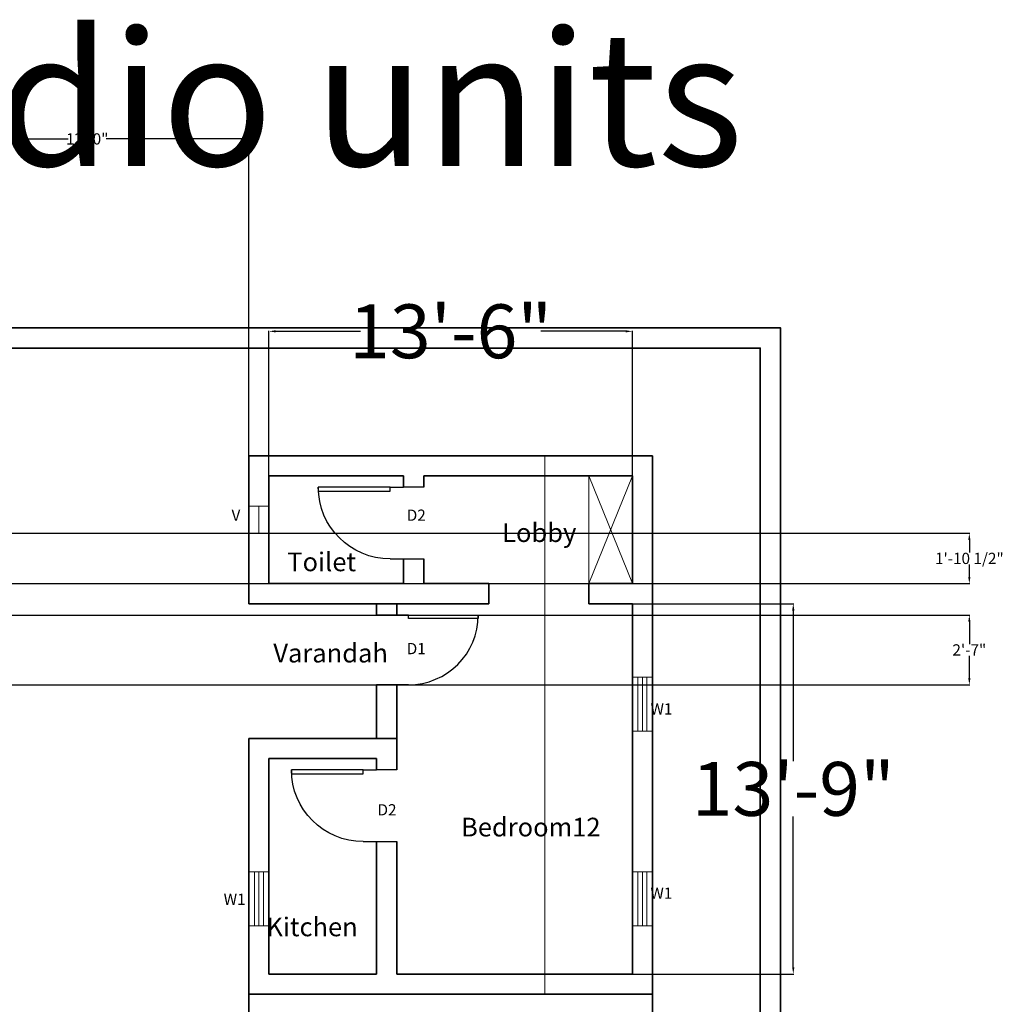
# Model space of a CAD drawing. Units: inches. Extents: x -205 to 674, y 63 to 1798.
# Tile 4 of 4: x 236 to 674, y 1359 to 1798. Entities that reach past the tile are written whole.
import ezdxf

# ---------------------------------------------------------------- set-up
doc = ezdxf.new("R2010")
doc.units = ezdxf.units.IN
doc.header["$MEASUREMENT"] = 0
doc.layers.get('0').update_dxf_attribs({"color": 70})
for name, color, linetype, lineweight in [('A-ANNO-DIMS', 240, 'Continuous', 18), ('A-ANNO-TEXT', 240, 'Continuous', 18), ('A-AREA-IDEN', 240, 'Continuous', 18), ('A-REFR', 8, 'Continuous', 13), ('A-WALL', 70, 'Continuous', 35), ('A-WALL-SITE', 70, 'Continuous', 35), ('door1', 20, 'Continuous', 25), ('door2', 160, 'Continuous', 25), ('lobby', 241, 'Continuous', 18), ('ventilator1', 210, 'Continuous', 18), ('window1', 50, 'Continuous', 18)]:
    doc.layers.add(name, color=color, linetype=linetype, lineweight=lineweight)
doc.styles.get("Standard").update_dxf_attribs({"font": 'arial.ttf'})
doc.dimstyles.get("Standard").update_dxf_attribs({"dimtxt": 5, "dimasz": 3, "dimexe": 0.18, "dimexo": 0.0625, "dimgap": 0.09, "dimtad": 0, "dimtih": 1, "dimtoh": 1, "dimdec": 0, "dimzin": 0, "dimdsep": 46, "dimlunit": 3, "dimtxsty": 'Standard', "dimcen": 0.09, "dimadec": 0, "dimazin": 0, "dimtfac": 1, "dimtdec": 0, "dimtofl": 0, "dimtmove": 0, "dimatfit": 3, "dimfxl": 1, "dimtolj": 1, "dimtzin": 0, "dimarcsym": 0})

# ---------------------------------------------------------------- blocks, each defined once
blk = doc.blocks.new('*D16')
at = {"layer": 'A-ANNO-DIMS', "color": 0, "lineweight": -2, "transparency": 16777216}
for p, q in [((509.6, 1537.3), (581.44, 1537.3)), ((581.26, 1534.3), (581.26, 1467.15)), ((581.26, 1375.3), (581.26, 1442.45)), ((509.6, 1372.3), (581.44, 1372.3))]:
    blk.add_line(p, q, dxfattribs=at)
at = {"layer": 'A-ANNO-DIMS', "color": 0, "transparency": 16777216}
for points in [[(580.76, 1534.3), (581.76, 1534.3), (581.26, 1537.3)], [(580.76, 1375.3), (581.76, 1375.3), (581.26, 1372.3)]]:
    blk.add_solid(points, dxfattribs=at)
at = {"layer": 'Defpoints', "color": 0, "transparency": 16777216}
for p in [(509.54, 1537.3), (509.54, 1372.3), (581.26, 1372.3)]:
    blk.add_point(p, dxfattribs=at)
at = {"layer": 'A-ANNO-DIMS', "color": 0, "transparency": 16777216, "insert": (581.26, 1454.8), "char_height": 5, "attachment_point": 5}
blk.add_mtext('\\A1;{\\H4.8x;13\'-9"}', dxfattribs=at)
blk = doc.blocks.new('*D17')
at = {"layer": 'A-ANNO-DIMS', "color": 0, "lineweight": -2, "transparency": 16777216}
for p, q in [((347.54, 1594.36), (347.54, 1658.92)), ((509.54, 1594.36), (509.54, 1658.92)), ((350.54, 1658.74), (388.36, 1658.74)), ((506.54, 1658.74), (468.73, 1658.74))]:
    blk.add_line(p, q, dxfattribs=at)
at = {"layer": 'A-ANNO-DIMS', "color": 0, "transparency": 16777216}
for points in [[(350.54, 1659.24), (350.54, 1658.24), (347.54, 1658.74)], [(506.54, 1659.24), (506.54, 1658.24), (509.54, 1658.74)]]:
    blk.add_solid(points, dxfattribs=at)
at = {"layer": 'Defpoints', "color": 0, "transparency": 16777216}
for p in [(347.54, 1658.74), (347.54, 1594.3), (509.54, 1594.3)]:
    blk.add_point(p, dxfattribs=at)
at = {"layer": 'A-ANNO-DIMS', "color": 0, "transparency": 16777216, "insert": (428.54, 1658.74), "char_height": 5, "attachment_point": 5}
blk.add_mtext('\\A1;{\\H4.8x;13\'-6"}', dxfattribs=at)
blk = doc.blocks.new('*U4')
for p, q in [((0, 0), (0, -6)), ((36, 0), (36, -6))]:
    blk.add_line(p, q)
blk.add_lwpolyline([(0, 0), (0, 36), (1.75, 36), (1.75, 0)], close=True)
blk.add_arc((0, 0), 36, 0, 90)
blk = doc.blocks.new('*U5')
for p, q in [((0, 0), (0, -6)), ((32, 0), (32, -6))]:
    blk.add_line(p, q)
blk.add_lwpolyline([(0, 0), (0, 32), (1.75, 32), (1.75, 0)], close=True)
blk.add_arc((0, 0), 32, 0, 90)
blk = doc.blocks.new('WIN-W1-24IN')
for p, q in [((2.5, 24), (2.5, 0)), ((4.5, 24), (4.5, 0)), ((6.5, 24), (6.5, 0))]:
    blk.add_line(p, q)
blk.add_lwpolyline([(0, 24), (9, 24), (9, 0), (0, 0)], close=True)
blk = doc.blocks.new('VENT-V-12IN')
blk.add_line((4.5, 12), (4.5, 0))
blk.add_lwpolyline([(9, 0), (0, 0), (0, 12), (9, 12)], close=True)
blk = doc.blocks.new('LOBBY-RECESS')
for p, q in [((0, 48), (19.36, 0)), ((0, 0), (19.36, 48)), ((19.36, 48), (19.36, 0))]:
    blk.add_line(p, q)
blk = doc.blocks.new('*D37')
at = {"layer": 'A-ANNO-DIMS', "color": 0, "lineweight": -2, "transparency": 16777216}
for p, q in [((194.54, 1603.36), (194.54, 1744.68)), ((197.54, 1744.5), (258.1, 1744.5)), ((335.54, 1744.5), (274.99, 1744.5)), ((338.54, 1603.36), (338.54, 1744.68))]:
    blk.add_line(p, q, dxfattribs=at)
at = {"layer": 'A-ANNO-DIMS', "color": 0, "transparency": 16777216}
for points in [[(197.54, 1745), (197.54, 1744), (194.54, 1744.5)], [(335.54, 1745), (335.54, 1744), (338.54, 1744.5)]]:
    blk.add_solid(points, dxfattribs=at)
at = {"layer": 'Defpoints', "color": 0, "transparency": 16777216}
for p in [(338.54, 1744.5), (194.54, 1603.3), (338.54, 1603.3)]:
    blk.add_point(p, dxfattribs=at)
at = {"layer": 'A-ANNO-DIMS', "color": 0, "transparency": 16777216, "insert": (266.54, 1744.5), "char_height": 5, "attachment_point": 5}
blk.add_mtext('\\A1;12\'-0"', dxfattribs=at)
blk = doc.blocks.new('*D43')
at = {"layer": 'A-ANNO-DIMS', "color": 0, "lineweight": -2, "transparency": 16777216}
for p, q in [((185.6, 1568.75), (659.92, 1568.75)), ((659.74, 1565.75), (659.74, 1560.2)), ((659.74, 1549.3), (659.74, 1554.85)), ((185.6, 1546.3), (659.92, 1546.3))]:
    blk.add_line(p, q, dxfattribs=at)
at = {"layer": 'A-ANNO-DIMS', "color": 0, "transparency": 16777216}
for points in [[(659.24, 1565.75), (660.24, 1565.75), (659.74, 1568.75)], [(659.24, 1549.3), (660.24, 1549.3), (659.74, 1546.3)]]:
    blk.add_solid(points, dxfattribs=at)
at = {"layer": 'Defpoints', "color": 0, "transparency": 16777216}
for p in [(185.54, 1568.75), (659.74, 1568.75), (185.54, 1546.3)]:
    blk.add_point(p, dxfattribs=at)
at = {"layer": 'A-ANNO-DIMS', "color": 0, "transparency": 16777216, "insert": (659.74, 1557.53), "char_height": 5, "attachment_point": 5}
blk.add_mtext('\\A1;1\'-10 1/2"', dxfattribs=at)
blk = doc.blocks.new('*D44')
at = {"layer": 'A-ANNO-DIMS', "color": 0, "lineweight": -2, "transparency": 16777216}
for p, q in [((137.6, 1532.3), (659.92, 1532.3)), ((659.74, 1529.3), (659.74, 1519.35)), ((659.74, 1504.19), (659.74, 1514.15)), ((137.6, 1501.19), (659.92, 1501.19))]:
    blk.add_line(p, q, dxfattribs=at)
at = {"layer": 'A-ANNO-DIMS', "color": 0, "transparency": 16777216}
for points in [[(659.24, 1529.3), (660.24, 1529.3), (659.74, 1532.3)], [(659.24, 1504.19), (660.24, 1504.19), (659.74, 1501.19)]]:
    blk.add_solid(points, dxfattribs=at)
at = {"layer": 'Defpoints', "color": 0, "transparency": 16777216}
for p in [(137.54, 1532.3), (137.54, 1501.19), (659.74, 1501.19)]:
    blk.add_point(p, dxfattribs=at)
at = {"layer": 'A-ANNO-DIMS', "color": 0, "transparency": 16777216, "insert": (659.74, 1516.75), "char_height": 5, "attachment_point": 5}
blk.add_mtext('\\A1;2\'-7"', dxfattribs=at)

msp = doc.modelspace()

# ---------------------------------------------------------------- linework, layer by layer
at = {"layer": 'A-REFR'}
msp.add_line((470.54, 1363.3), (470.54, 1603.3), dxfattribs=at)
at = {"layer": 'A-WALL'}
for p, q in [((518.54, 1603.3), (338.54, 1603.3)), ((338.54, 1603.3), (338.54, 1537.3)), ((518.54, 1363.3), (518.54, 1603.3)), ((407.54, 1594.3), (347.54, 1594.3)), ((347.54, 1594.3), (347.54, 1546.3)), ((407.54, 1594.3), (407.54, 1589.3)), ((407.54, 1594.3), (407.54, 1589.3)), ((509.54, 1594.3), (416.54, 1594.3)), ((416.54, 1594.3), (416.54, 1589.3)), ((416.54, 1589.3), (416.54, 1594.3)), ((509.54, 1546.3), (509.54, 1594.3)), ((407.54, 1557.3), (407.54, 1546.3)), ((416.54, 1557.3), (416.54, 1546.3)), ((407.54, 1546.3), (347.54, 1546.3)), ((445.59, 1546.3), (416.54, 1546.3)), ((445.59, 1546.3), (445.59, 1537.3)), ((509.54, 1546.3), (490.18, 1546.3)), ((490.18, 1546.3), (490.18, 1537.3)), ((445.59, 1537.3), (338.54, 1537.3)), ((395.54, 1537.3), (395.54, 1532.3)), ((395.54, 1537.29), (395.54, 1532.4)), ((404.54, 1537.3), (404.54, 1532.3)), ((445.59, 1537.3), (445.59, 1537.3)), ((509.54, 1537.3), (490.18, 1537.3)), ((490.18, 1537.3), (490.18, 1537.3)), ((509.54, 1372.3), (509.54, 1537.3)), ((395.54, 1501.19), (395.54, 1477.3)), ((404.54, 1501.19), (404.54, 1463.3)), ((338.54, 1477.3), (338.54, 1363.3)), ((338.54, 1477.3), (404.54, 1477.3)), ((347.54, 1468.3), (347.54, 1372.3)), ((347.54, 1468.3), (395.54, 1468.3)), ((395.54, 1468.3), (395.54, 1463.3)), ((395.54, 1468.3), (395.54, 1463.3)), ((404.54, 1463.3), (404.54, 1468.3)), ((395.54, 1431.3), (395.54, 1372.3)), ((395.54, 1431.3), (395.54, 1372.3)), ((404.54, 1431.3), (404.54, 1372.3)), ((347.54, 1372.3), (395.54, 1372.3)), ((404.54, 1372.3), (509.54, 1372.3)), ((338.54, 1363.3), (518.54, 1363.3)), ((338.54, 1249.3), (338.54, 1363.3)), ((338.54, 1363.3), (518.54, 1363.3)), ((518.54, 1363.3), (518.54, 1123.3))]:
    msp.add_line(p, q, dxfattribs=at)
at = {"layer": 'A-WALL-SITE'}
for points in [[(575.54, 154.3), (575.54, 1660.3), (266.54, 1660.3), (-42.46, 1660.3), (-42.46, 154.3), (266.54, 154.3)], [(566.54, 163.3), (566.54, 1651.3), (266.54, 1651.3), (-33.46, 1651.3), (-33.46, 163.3), (266.54, 163.3)]]:
    msp.add_lwpolyline(points, close=True, dxfattribs=at)
at = {"layer": 'door1'}
for p, q in [((404.54, 1532.3), (395.54, 1532.3)), ((404.54, 1501.19), (395.54, 1501.19))]:
    msp.add_line(p, q, dxfattribs=at)
at = {"layer": 'door2'}
for p, q in [((416.54, 1589.3), (407.54, 1589.3)), ((407.54, 1557.3), (416.54, 1557.3)), ((404.54, 1463.3), (395.54, 1463.3)), ((395.54, 1431.3), (404.54, 1431.3))]:
    msp.add_line(p, q, dxfattribs=at)

# ---------------------------------------------------------------- block references
at = {"layer": 'door1', "xscale": 0.8640557789234337, "yscale": 0.8640557789234337, "zscale": 0.8640557789234337, "rotation": 270}
msp.add_blockref('*U4', (409.73, 1532.3), dxfattribs=at)
at = {"layer": 'door2', "xscale": -1, "rotation": 90}
for p in [(401.54, 1589.3), (389.54, 1463.3)]:
    msp.add_blockref('*U5', p, dxfattribs=at)
at = {"layer": 'lobby', "rotation": 180}
msp.add_blockref('LOBBY-RECESS', (509.54, 1594.3), dxfattribs=at)
at = {"layer": 'ventilator1', "extrusion": (0, 0, -1), "zscale": -1}
msp.add_blockref('VENT-V-12IN', (-347.54, 1568.75), dxfattribs=at)
at = {"layer": 'window1', "extrusion": (0, 0, -1), "zscale": -1}
for p in [(-518.54, 1480.57), (-347.54, 1393.81), (-518.54, 1393.81)]:
    msp.add_blockref('WIN-W1-24IN', p, dxfattribs=at)

# ---------------------------------------------------------------- texts
at = {"layer": 'A-ANNO-TEXT'}
for s, width, insert, char_height, attachment_point in [('Studio units', 509.5824, (97.11, 1792.47), 60, 1), ('V', 13.5017, (334.78, 1579.29), 5, 3), ('D2', 13.5017, (417.45, 1579.29), 5, 3), ('D1', 13.5017, (417.45, 1519.84), 5, 3), ('W1', 13.5017, (527.4, 1492.96), 5, 3), ('D2', 13.5017, (404.41, 1447.99), 5, 3), ('W1', 13.5017, (527.34, 1410.83), 5, 3), ('W1', 13.5017, (337.12, 1408.11), 5, 3)]:
    msp.add_mtext_dynamic_manual_height_columns(s, width=width, gutter_width=1, heights=[0], dxfattribs=dict(at, insert=insert, char_height=char_height, attachment_point=attachment_point))
at = {"layer": 'A-AREA-IDEN', "char_height": 8.34, "attachment_point": 3}
for s, insert in [('Lobby', (484.55, 1573.17)), ('Toilet', (386.37, 1560.16)), ('Varandah', (400.56, 1519.49)), ('Bedroom12', (495.36, 1441.95)), ('Kitchen', (387.1, 1397.47))]:
    msp.add_mtext_dynamic_manual_height_columns(s, width=37.3149, gutter_width=1.67, heights=[0], dxfattribs=dict(at, insert=insert))

# ---------------------------------------------------------------- dimensions: what is measured, and where the dimension line sits
at = {"layer": 'A-ANNO-DIMS'}
dim = msp.add_linear_dim(base=(338.54, 1744.5), p1=(194.54, 1603.3), p2=(338.54, 1603.3), dimstyle='Standard', override={"dimdec": 1, "dimlfac": 1, "dimrnd": 0, "dimzin": 1, "dimdsep": 46, "dimlunit": 4, "dimfrac": 2}, dxfattribs=at)
dim.commit()
dim.dimension.update_dxf_attribs({"geometry": '*D37', "text_midpoint": (266.54, 1744.5)})
for base, p1, p2, angle, picture, middle in [((347.54, 1658.74), (509.54, 1594.3), (347.54, 1594.3), 180, '*D17', (428.54, 1658.74)), ((581.26, 1372.3), (509.54, 1537.3), (509.54, 1372.3), 90, '*D16', (581.26, 1454.8))]:
    dim = msp.add_linear_dim(base=base, p1=p1, p2=p2, angle=angle, text='{\\H4.8x;<>}', dimstyle='Standard', override={"dimclrd": 0, "dimclre": 0, "dimclrt": 0}, dxfattribs=at)
    dim.commit()
    dim.dimension.update_dxf_attribs({"geometry": picture, "text_midpoint": middle})
for base, p1, p2, picture, middle in [((659.7424, 1568.7532), (185.5424, 1546.2998), (185.5424, 1568.7532), '*D43', (659.7424, 1557.5265)), ((659.74, 1501.19), (137.54, 1532.3), (137.54, 1501.19), '*D44', (659.74, 1516.75))]:
    dim = msp.add_linear_dim(base=base, p1=p1, p2=p2, angle=90, dimstyle='Standard', override={"dimdec": 1, "dimlfac": 1, "dimrnd": 0, "dimzin": 1, "dimdsep": 46, "dimlunit": 4, "dimfrac": 2}, dxfattribs=at)
    dim.commit()
    dim.dimension.update_dxf_attribs({"geometry": picture, "text_midpoint": middle})

doc.saveas('drawing.dxf')
